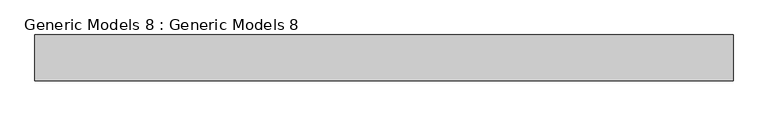
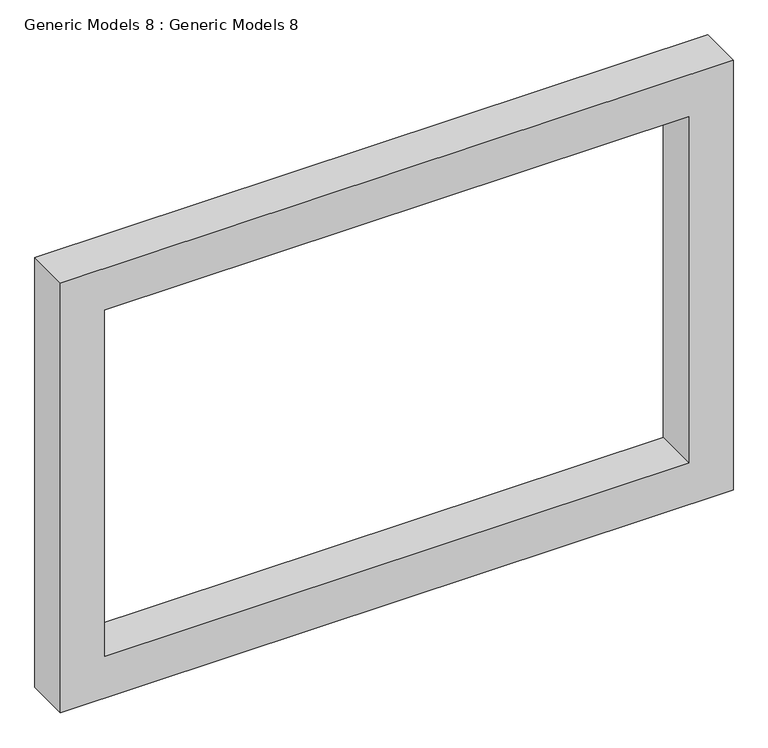
"""IFC4 building model written with IfcOpenShell, lengths in millimetres: proxy geometry, Generic Models 8 : Generic Models 8."""

from ifc_helpers import new_model, si_unit, frame, origin, place, context, project, spatial, polyline, outline, extrude, source, transform, mapped, element, save


def generic_models_8_generic_models_8_56cf2c1e(model_context):
    return source(origin(), model_context, "Body", "SweptSolid", [
        extrude(outline(polyline([(2717.2, -2922.9474631), (1152.4, -2922.9474631), (1152.4, -608.1474631), (2717.2, -608.1474631), (2717.2, -2922.9474631)]), holes=[polyline([(2564.8, -2770.5474631), (2564.8, -760.5474631), (1304.8, -760.5474631), (1304.8, -2770.5474631), (2564.8, -2770.5474631)])]), frame((0.0, 10129.5061648, 0.0), z_axis=(0.0, 1.0, 0.0), x_axis=(0.0, 0.0, 1.0)), (0.0, 0.0, 1.0), 152.4),
    ])


if __name__ == "__main__":
    model = new_model("IFC4")
    model_context = context("Model", 3, world=origin())
    ifc_project = project(units=[si_unit("LENGTHUNIT", "METRE", prefix="MILLI")], contexts=[model_context])
    site = spatial("IfcSite", under=ifc_project)
    building = spatial("IfcBuilding", under=site)
    placement = place(None, origin())
    generic_models_8_generic_models_8_shape = generic_models_8_generic_models_8_56cf2c1e(model_context)
    element("IfcBuildingElementProxy", 1, Name="Generic Models 8 : Generic Models 8", ObjectType="Generic Models 8 : Generic Models 8", at=placement, inside=building, context=model_context, shape_type="MappedRepresentation", body=[
        mapped(generic_models_8_generic_models_8_shape, transform((0.0, 0.0, 0.0), x_axis=(1.0, 0.0, 0.0), y_axis=(0.0, 1.0, 0.0), z_axis=(0.0, 0.0, 1.0))),
    ])
    save(model, "model.ifc")

# Revit data of these elements
# Element 1 (IfcBuildingElementProxy, "Generic Models 8 : Generic Models 8")
#   Materials on its faces: "WALL PAINT"
# Materials
#   "WALL PAINT": class "Generic", colour RGB 120 120 120, transparency 0, Cost = 0
